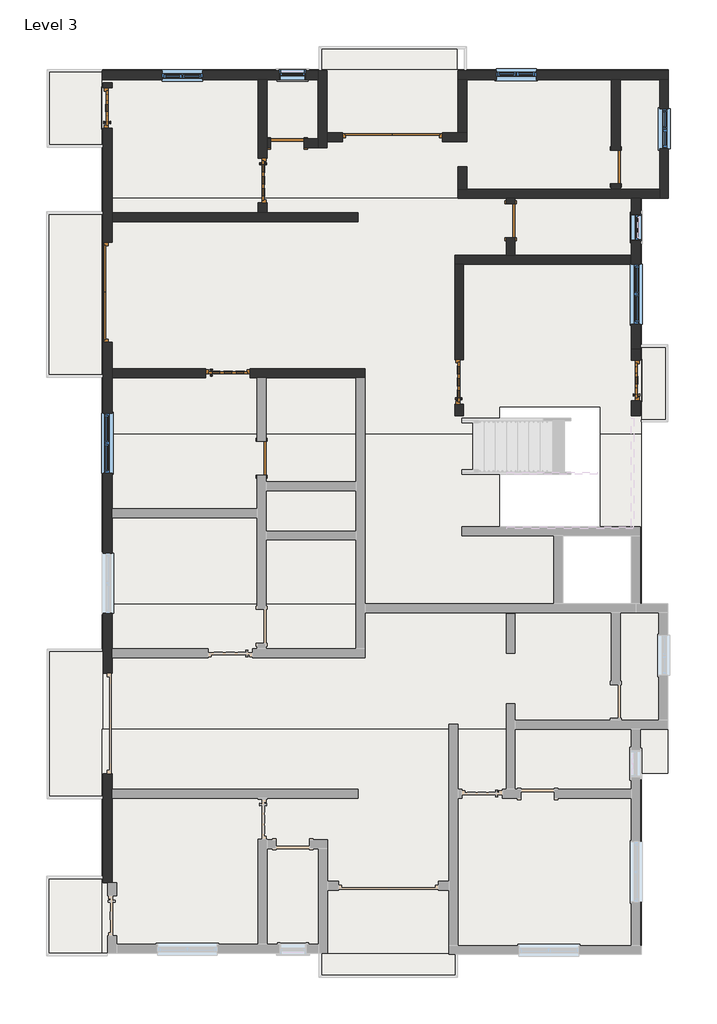
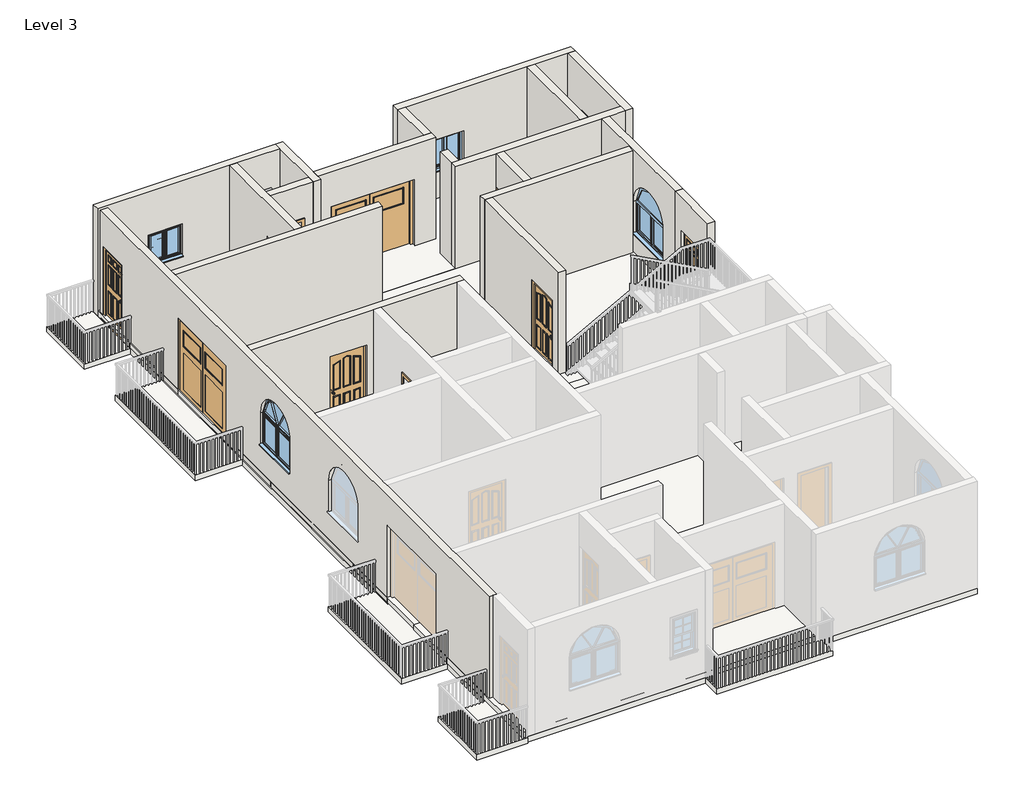
# One storey, part 2 of 7: 19 walls, 11 doors, 10 slabs, 7 windows, 5 roofs.
# Revit data of these elements (continued)
# Type "Windows_Dbl_w-Glazing_Bars : 910x910mm" (continued)
#   Window Board Extension = 0' - 0.98425"
#   Visual Light Transmittance = 0.9
#   Solar Heat Gain Coefficient = 0.78
#   Rough Width = 2' - 11.82677"
#   Rough Height = 2' - 11.82677"
#   Height = 2' - 11.82677"
#   Width = 2' - 11.82677"
#   Heat Transfer Coefficient (U) = 0.6496 BTU/(h·ft²·°F)
#   Glazing Thickness = 0' - 0.94488"
#   Glazing Bar Thickness = 0' - 0.7874"
#   FrameOffset - External = 0' - 1.9685"
#   Frame Depth = 0' - 2.55906"
#   Default Head Height = 6' - 10.67717"
#   Cill Depth = 0' - 3.44488"
#   Cavity Closer Width = 0' - 1.9685"
#   Cavity Closer Offset from Ext = 0' - 4.03543"
#   Cavity Closer Depth = 0' - 3.34646"
#   Vis - Glazing Bars = yes
#   Vis - Cavity Closers = yes
#   Define Thermal Properties by = 1
#   Material Trim = Window Frame
#   Material Glazing Bars = Window Frame
#   Material Glass = Glass
#   Material Frame = Window Frame
#   Wall Closure = (empty or 0)
# Elements 1, 2 (IfcDoor, "Doors_ExtSgl_5 : 910x2110mm")
#   Phase Created = New Construction
#   Materials on its faces: "Door - Panel", "Door - Handle", "Door - Frame/Mullion", "Door - Glazing"
# Elements 3, 4, 5 (IfcDoor, "Doors_ExtSgl_6 : 1010x2110mm")
#   Phase Created = New Construction
#   Materials on its faces: "Door - Panel", "Door - Handle", "Door - Frame/Mullion", "Door - Glazing"
# Element 6 (IfcDoor, "Doors_Garage_Timber_Side_Hung_Glazing : 2270x2050mm")
#   Phase Created = New Construction
#   Materials on its faces: "Door - Panel", "Door - Frame/Mullion", "Door - Glazing"
# Element 7 (IfcDoor, "Doors_Garage_Timber_Side_Hung_Glazing : 2270x2200mm")
#   Phase Created = New Construction
#   Materials on its faces: "Door - Panel", "Door - Frame/Mullion", "Door - Glazing"
# Elements 8, 9, 10, 11 (IfcDoor, "Single-Flush : 30\" x 80\"")
#   Phase Created = New Construction
#   Materials on its faces: "Door - Frame", "Door - Panel"
# Elements 12, 16 (IfcRoof, "Generic - 12\"")
#   built-in parameter 1001705 = 20.5 (stored number, unit not read)
#   built-in parameter 1001710 = 33615
#   Phase Created = New Construction
#   Materials on its faces: "Default Roof", "Earth"
# Elements 13, 14 (IfcRoof, "Generic - 12\"")
#   built-in parameter 1001705 = 20.5 (stored number, unit not read)
#   built-in parameter 1001710 = 33615
#   Phase Created = New Construction
#   Materials on its faces: "Default Roof"
# Element 15 (IfcRoof, "Generic - 12\"")
#   built-in parameter 1001705 = 20.5 (stored number, unit not read)
#   built-in parameter 1001710 = 33615
#   Phase Created = New Construction
#   Materials on its faces: "Default Roof", "Wood - Stained"
# Element 17 (IfcSlab, "Generic - 12\"")
#   Height Offset From Level = 0' - 0"
#   Phase Created = New Construction
#   Materials on its faces: "Default Floor", "Concrete, Lightweight"
# Element 18 (IfcSlab, "Generic - 12\"")
#   Height Offset From Level = 0' - 0"
#   Phase Created = New Construction
#   Materials on its faces: "Default Floor", "Wood - Stained", "Earth", "Concrete, Lightweight"
# Elements 19, 21, 22, 23, 24, 25 (IfcSlab, "Generic - 12\"")
#   Height Offset From Level = 0' - 0"
#   Phase Created = New Construction
#   Materials on its faces: "Default Floor"
# Element 20 (IfcSlab, "Generic - 12\"")
#   Height Offset From Level = 0' - 0"
#   Phase Created = New Construction
#   Materials on its faces: "Default Floor", "mm"
# Element 26 (IfcSlab, "Generic - 12\"")
#   Height Offset From Level = 0' - 0"
#   Phase Created = New Construction
#   Materials on its faces: "Default Floor", "Earth"
# Elements 27, 31 (IfcWall, "Generic - 9\" w")
#   Top Offset = 0' - 0"
#   Base Offset = 0' - 0"
#   wall height = 10' - 0"
#   Phase Created = New Construction
#   Base Constraint = Level 3
#   Top Constraint = Level 4
#   Materials on its faces: "Default Wall", "Earth"
# Element 28 (IfcWall, "Generic - 9\" w")
#   Top Offset = 0' - 0"
#   Base Offset = 0' - 0"
#   wall height = 10' - 0"
#   Phase Created = New Construction
#   Base Constraint = Level 3
#   Top Constraint = Level 4
#   Materials on its faces: "Default Wall", "Wood - Stained"
# Element 29 (IfcWall, "Generic - 9\" w")
#   Top Offset = 0' - 0"
#   Base Offset = 0' - 0"
#   wall height = 10' - 0"
#   Phase Created = New Construction
#   Base Constraint = Level 3
#   Top Constraint = Level 4
#   Materials on its faces: "Default Wall", "Grass"
# Element 30 (IfcWall, "Generic - 9\" w")
#   Top Offset = 0' - 0"
#   Base Offset = 0' - 0"
#   wall height = 10' - 0"
#   Phase Created = New Construction
#   Base Constraint = Level 3
#   Top Constraint = Level 4
#   Materials on its faces: "Default Wall", "mm"
# Elements 32, 33, 35, 37, 38, 40, 41, 42, 43, 44, 45 (IfcWall, "Generic -4.5\" p")
#   Top Offset = 0' - 0"
#   Base Offset = 0' - 0"
#   wall height = 10' - 0"
#   Phase Created = New Construction
#   Base Constraint = Level 3
#   Top Constraint = Level 4
#   Materials on its faces: "Default Wall"
# Elements 34, 39 (IfcWall, "Generic -4.5\" p")
#   Top Offset = 0' - 0"
#   Base Offset = 0' - 0"
#   wall height = 10' - 0"
#   Phase Created = New Construction
#   Base Constraint = Level 3
#   Top Constraint = Level 4
#   Materials on its faces: "Default Wall", "Earth"
# Element 36 (IfcWall, "Generic -4.5\" p")
#   Top Offset = 0' - 0"
#   Base Offset = 0' - 0"
#   wall height = 10' - 0"
#   Phase Created = New Construction
#   Base Constraint = Level 3
#   Top Constraint = Level 4
#   Materials on its faces: "Default Wall", "Oak Flooring"
# Element 46 (IfcWindow, "Window-Double-Hung : 24\" x 42\"")
#   Mark = "36"
#   Window Inset = 0' - 0"
#   Interior Wall Closure = 0' - 1 1/2"
#   Frame Extension = 0' - 1 1/4"
#   Exterior Wall Closure = 0' - 0 1/2"
#   Interior Trim Visibility = yes
#   Indicator Visibility = yes
#   Exterior Trim Visibility = yes
#   Phase Created = New Construction
#   Materials on its faces: "Wood - Stained", "Glass", "Clad - White"
# Element 47 (IfcWindow, "Window-Double-Hung : 24\" x 42\"")
#   Mark = "42"
#   Window Inset = 0' - 0"
#   Interior Wall Closure = 0' - 1 1/2"
#   Frame Extension = 0' - 1 1/4"
#   Exterior Wall Closure = 0' - 0 1/2"
#   Interior Trim Visibility = yes
#   Indicator Visibility = yes
#   Exterior Trim Visibility = yes
#   Phase Created = New Construction
#   Materials on its faces: "Wood - Stained", "Glass", "Clad - White"
# Element 48 (IfcWindow, "Windows_Arched : 1360x910mm")
#   Mark = "32"
#   Phase Created = New Construction
#   Materials on its faces: "Window Frame", "Glass"
# Element 49 (IfcWindow, "Windows_Arched : 1360x910mm")
#   Mark = "43"
#   Phase Created = New Construction
#   Materials on its faces: "Window Frame", "Glass"
# Element 50 (IfcWindow, "Windows_Dbl_w-Glazing_Bars : 910x910mm")
#   Mark = "39"
#   Phase Created = New Construction
#   Materials on its faces: "Window Frame", "Glass"
# Element 51 (IfcWindow, "Windows_Dbl_w-Glazing_Bars : 910x910mm")
#   Mark = "40"
#   Phase Created = New Construction
#   Materials on its faces: "Window Frame", "Glass"
# Element 52 (IfcWindow, "Windows_Dbl_w-Glazing_Bars : 910x910mm")
#   Mark = "41"
#   Phase Created = New Construction
#   Materials on its faces: "Window Frame", "Glass"
# Materials
#   "Door - Glazing": colour RGB 0 0 255, transparency 0.75
#   "Door - Panel": class "Wood", colour RGB 210 159 95, transparency 0, Cost = 0
#   "Door - Frame/Mullion": class "Wood", colour RGB 212 179 113, transparency 0
#   "Door - Handle": colour RGB 0 0 0, transparency 0
#   "Door - Frame": colour RGB 118 70 51, transparency 0, Cost = 0
#   "Wood - Stained": class "Wood", colour RGB 224 178 126, transparency 0, Cost = 0
#   "Clad - White": class "Wood", colour RGB 242 242 238, transparency 0, Cost = 0
#   "Glass": class "Glass", colour RGB 0 128 192, transparency 0.75, Description = "Soda Lime Glass", Cost = 0
#   "Window Frame": colour RGB 249 249 249, transparency 0
#   "Default Roof": colour RGB 88 101 114, transparency 0, Cost = 0
#   "Earth": class "Generic", colour RGB 97 75 62, transparency 0, Description = "Soil", Cost = 0
#   "Default Floor": colour RGB 128 128 128, transparency 0, Cost = 0
#   "Concrete, Lightweight": class "Concrete", colour RGB 142 141 140, transparency 0, Description = "Lightweight concrete", Cost = 0
#   "mm": class "Generic", colour RGB 128 64 0, transparency 0.5, Cost = 0
#   "Default Wall": colour RGB 128 128 128, transparency 0, Cost = 0
#   "Grass": class "Generic", colour RGB 104 137 66, transparency 0, Description = "Physical material.", Cost = 0
#   "Oak Flooring": class "Wood", colour RGB 216 169 114, transparency 0, Description = "Quercus Rubra", Cost = 0
